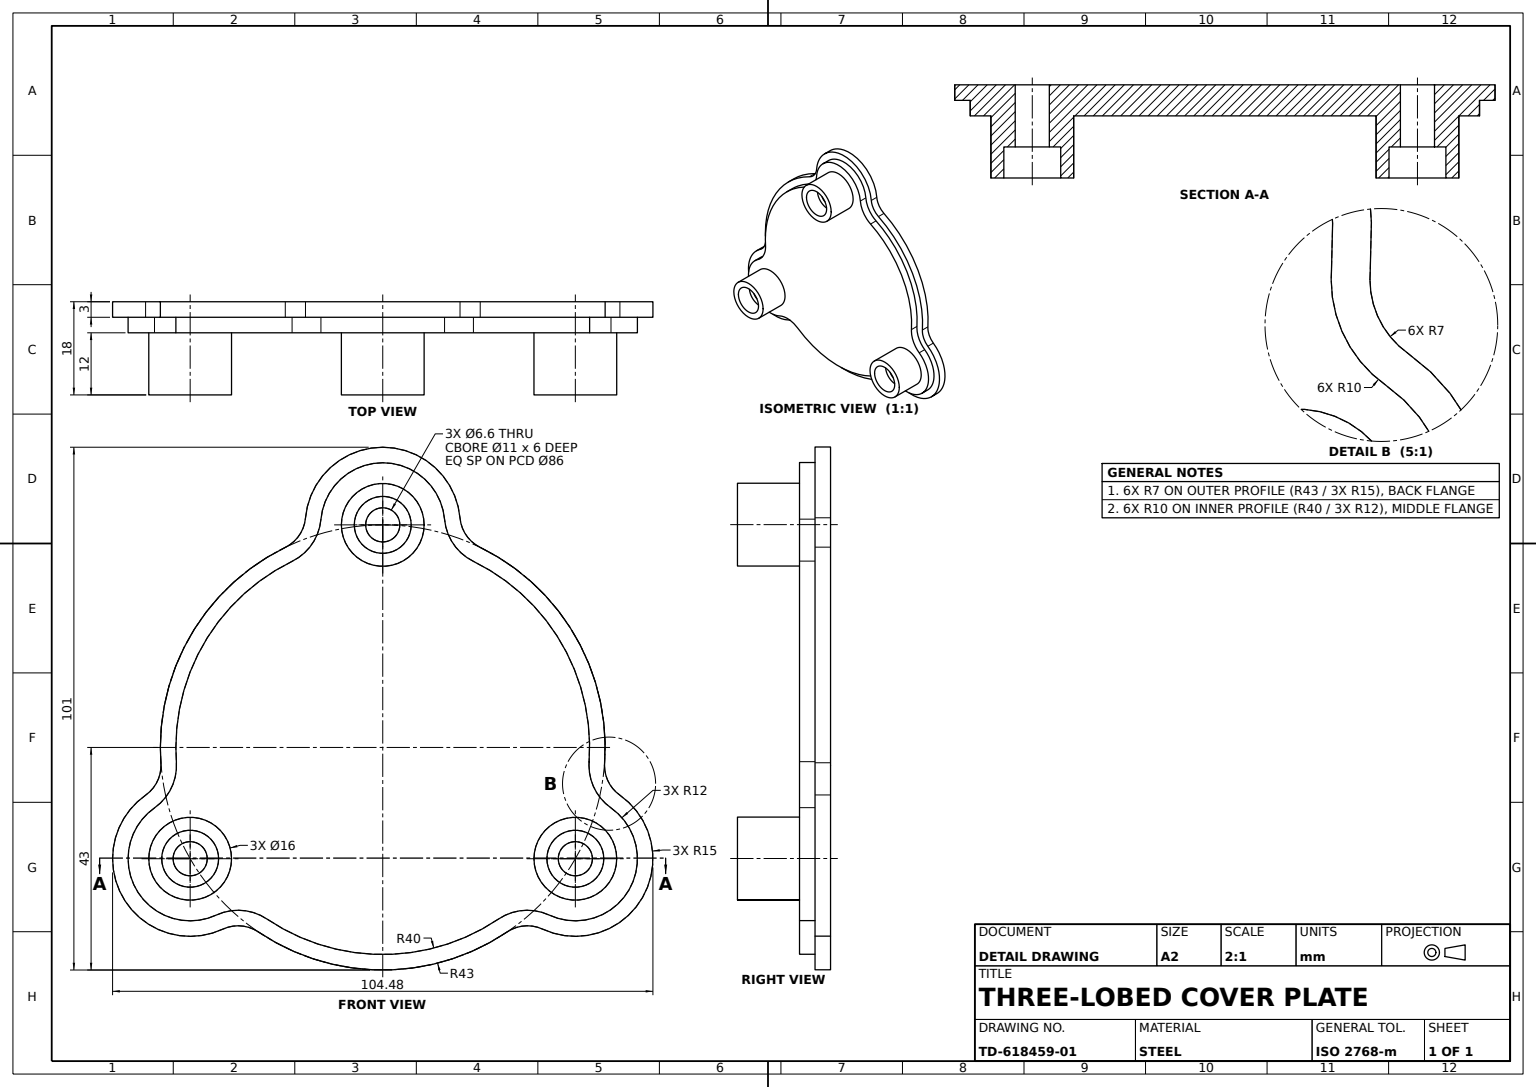
from build123d import *

# Parameters (mm, degrees)
BASE_PLATE_3MM_DEPTH              = 3
RAISED_STEP_3MM_DEPTH             = 3
BOSS_PROFILE_3X_16_R              = 8
BOSSES_3X_16X12_DEPTH             = 12
COUNTERBORE_PROFILE_3X_11_R       = 5.5
COUNTERBORES_3X_11X6_DEPTH        = 6
CLEARANCE_HOLE_PROFILE_3X_6_6_R   = 3.3
CLEARANCE_HOLES_3X_6_6_THRU_DEPTH = 146


with BuildPart() as part:
    # Base Plate Profile → Base Plate 3mm (new body)
    with BuildSketch(Plane.XY):
        with BuildLine():
            ThreePointArc((-18.846153454, 38.65), (-37.239092363, 21.5), (-42.894958583, -3.003752345))
            ThreePointArc((-42.894958583, -3.003752345), (-43.557934635, -6.502479184), (-45.856433127, -9.222319513))
            ThreePointArc((-45.856433127, -9.222319513), (-50.229473419, -29), (-30.914979544, -35.101676259))
            ThreePointArc((-30.914979544, -35.101676259), (-27.410279478, -34.471038339), (-24.048805129, -35.646247655))
            ThreePointArc((-24.048805129, -35.646247655), (0, -43), (24.048805129, -35.646247655))
            ThreePointArc((24.048805129, -35.646247655), (27.410279478, -34.471038339), (30.914979544, -35.101676259))
            ThreePointArc((30.914979544, -35.101676259), (50.22947342, -29), (45.856433127, -9.222319513))
            ThreePointArc((45.856433127, -9.222319513), (43.557934635, -6.502479184), (42.894958583, -3.003752345))
            ThreePointArc((42.894958583, -3.003752345), (37.239092363, 21.5), (18.846153454, 38.65))
            ThreePointArc((18.846153454, 38.65), (16.147655157, 40.973517522), (14.941453584, 44.323995772))
            ThreePointArc((14.941453584, 44.323995772), (0, 58), (-14.941453584, 44.323995772))
            ThreePointArc((-14.941453584, 44.323995772), (-16.147655157, 40.973517522), (-18.846153454, 38.65))
        make_face()
    extrude(amount=BASE_PLATE_3MM_DEPTH)

    # Raised Step Profile → Raised Step 3mm (add)
    with BuildSketch(Plane.XY.offset(3)):
        with BuildLine():
            ThreePointArc((-17.531305538, 35.953488372), (-13.676307972, 39.272799119), (-11.953162867, 44.059196617))
            ThreePointArc((-11.953162867, 44.059196617), (0, 55), (11.953162867, 44.059196617))
            ThreePointArc((11.953162867, 44.059196617), (13.676307972, 39.272799119), (17.531305538, 35.953488372))
            ThreePointArc((17.531305538, 35.953488372), (34.641016151, 20), (39.902287054, -2.794188228))
            ThreePointArc((39.902287054, -2.794188228), (40.8493957, -7.792369426), (44.132964974, -11.67785561))
            ThreePointArc((44.132964974, -11.67785561), (47.631397208, -27.5), (32.179802107, -32.381341007))
            ThreePointArc((32.179802107, -32.381341007), (27.173087728, -31.480429693), (22.370981516, -33.159300144))
            ThreePointArc((22.370981516, -33.159300144), (0, -40), (-22.370981516, -33.159300144))
            ThreePointArc((-22.370981516, -33.159300144), (-27.173087728, -31.480429693), (-32.179802107, -32.381341007))
            ThreePointArc((-32.179802107, -32.381341007), (-47.631397208, -27.5), (-44.132964974, -11.67785561))
            ThreePointArc((-44.132964974, -11.67785561), (-40.8493957, -7.792369426), (-39.902287054, -2.794188228))
            ThreePointArc((-39.902287054, -2.794188228), (-34.641016151, 20), (-17.531305538, 35.953488372))
        make_face()
    extrude(amount=RAISED_STEP_3MM_DEPTH)

    # Boss Profile 3xØ16 → Bosses 3xØ16x12 (add)
    with BuildSketch(Plane.XY.offset(6)):
        with Locations((0, 43)):
            Circle(BOSS_PROFILE_3X_16_R)
        with Locations((37.239092363, -21.5)):
            Circle(BOSS_PROFILE_3X_16_R)
        with Locations((-37.239092363, -21.5)):
            Circle(BOSS_PROFILE_3X_16_R)
    extrude(amount=BOSSES_3X_16X12_DEPTH)

    # Counterbore Profile 3xØ11 → Counterbores 3xØ11x6 (cut)
    with BuildSketch(Plane.XY.offset(18)):
        with Locations((0, 43)):
            Circle(COUNTERBORE_PROFILE_3X_11_R)
        with Locations((37.239092363, -21.5)):
            Circle(COUNTERBORE_PROFILE_3X_11_R)
        with Locations((-37.239092363, -21.5)):
            Circle(COUNTERBORE_PROFILE_3X_11_R)
    extrude(amount=-COUNTERBORES_3X_11X6_DEPTH, mode=Mode.SUBTRACT)

    # Clearance Hole Profile 3xØ6.6 → Clearance Holes 3xØ6.6 Thru (cut)
    with BuildSketch(Plane.XY.offset(12)):
        with Locations((0, 43)):
            Circle(CLEARANCE_HOLE_PROFILE_3X_6_6_R)
        with Locations((37.239092363, -21.5)):
            Circle(CLEARANCE_HOLE_PROFILE_3X_6_6_R)
        with Locations((-37.239092363, -21.5)):
            Circle(CLEARANCE_HOLE_PROFILE_3X_6_6_R)
    extrude(amount=-CLEARANCE_HOLES_3X_6_6_THRU_DEPTH, mode=Mode.SUBTRACT)


solid = part.part
